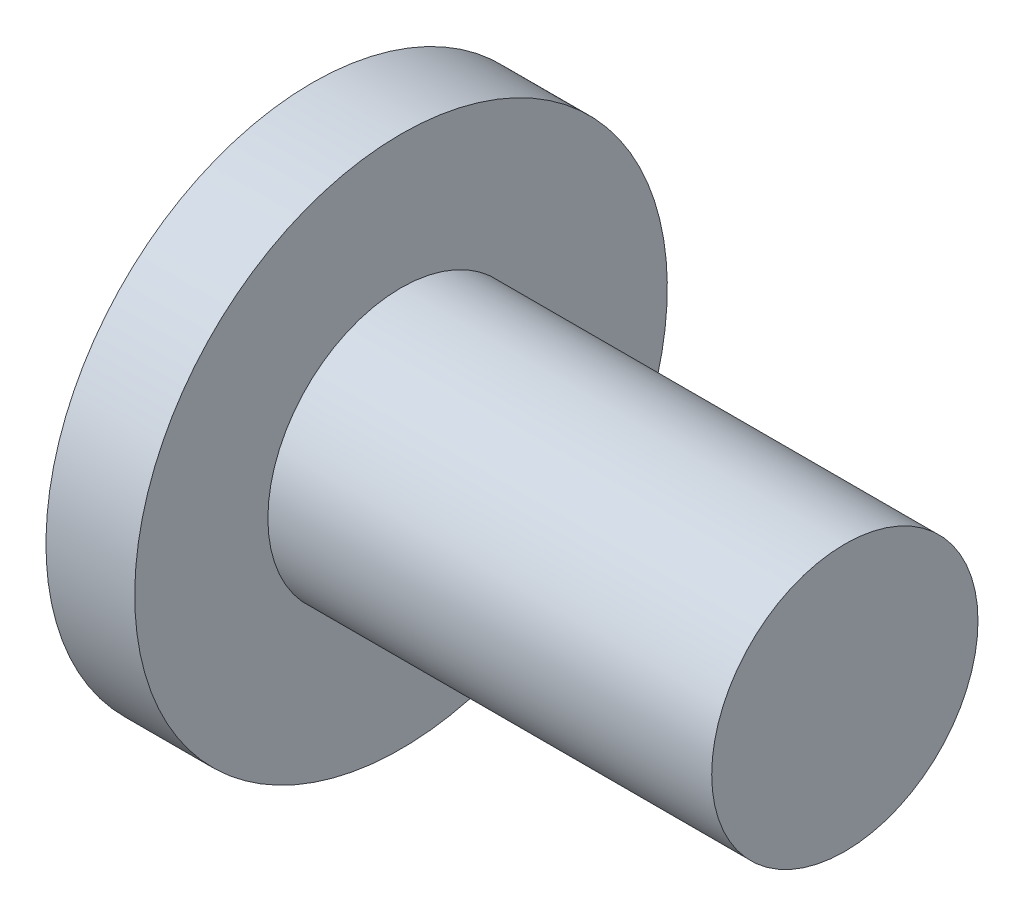
SolidWorks part; units mm, degrees
material "Plain Carbon Steel"
ref_plane "Front Plane" through (0, 0, 0) normal (0, 0, 1) x (1, 0, 0)
ref_plane "Top Plane" through (0, 0, 0) normal (0, 1, 0) x (1, 0, 0)
ref_plane "Right Plane" through (0, 0, 0) normal (1, 0, 0) x (0, 0, -1)
sketch "Pin Profile Sketch" plane through (0, 0, 0) normal (0, 0, 1) x (1, 0, 0)
  line L0 (0, 0) -> (-12, 0)
  line L1 (-12, 0) -> (-12, 6)
  line L2 (-12, 6) -> (-10, 6)
  line L3 (-10, 6) -> (-10, 3)
  line L4 (-10, 3) -> (0, 3)
  line L5 (0, 3) -> (0, 0)
  dimension "D1" = 3
  dimension "D2" = 10
  dimension "D3" = 2
  dimension "D4" = 6
revolve "Headed Pin Revolve" add sketch "Pin Profile Sketch" angle 360 about L0
